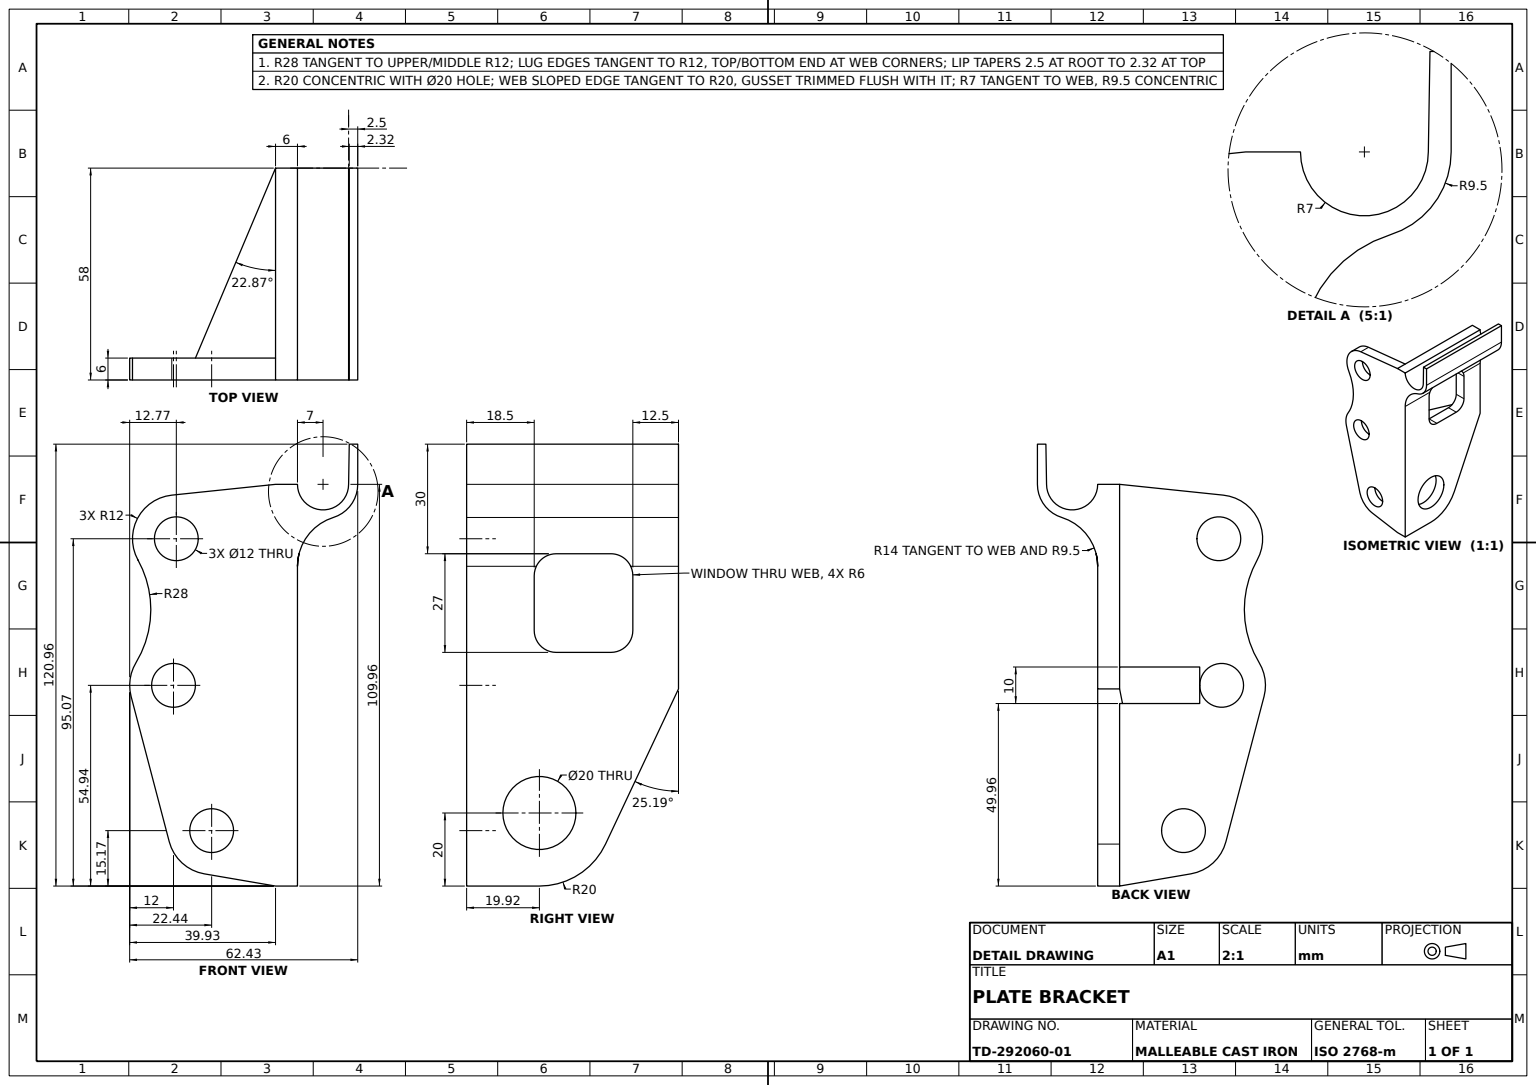
SolidWorks part; units mm, degrees
material "Malleable Cast Iron"
ref_plane "Front Plane" through (0, 0, 0) normal (0, 0, 1) x (1, 0, 0)
ref_plane "Top Plane" through (0, 0, 0) normal (0, 1, 0) x (1, 0, 0)
ref_plane "Right Plane" through (0, 0, 0) normal (1, 0, 0) x (0, 0, -1)
sketch "Base Plate Sketch" plane through (0, 0, 0) normal (0, 0, 1) x (1, 0, 0)
  line L0 (0, 0) -> (58, 0)
  line L1 (58, 0) -> (58, -56)
  line L2 (0, 0) -> (0, -56)
  line L3 (0, -56) -> (58, -56)
  dimension "D1" = 56
  dimension "D2" = 58
extrude "Base Plate" add sketch "Base Plate Sketch" along normal blind 6
sketch "Channel Wall Sketch" plane through (0, 0, 0) normal (-1, 0, 0) x (0, 0, 1)
  line L0 (0, 0) -> (-7, 0)
  line L1 (0, 0) -> (0, -56) construction
  line L2 (-7, 0) -> (-16.5, 0)
  line L3 (0, 0) -> (0, -22.4332)
  arc A1 (-16.5, 0) -> (-9.8298, -9.0688) centre (-7, 0) ccw
  arc A2 (-9.8298, -9.0688) -> (0, -22.4332) centre (-14, -22.4332) cw
  dimension "D2" = 19
  dimension "D3" = 14
  dimension "D4" = 19
  dimension "D7" = 14
  dimension "D6" = 7
extrude "Channel Wall" add sketch "Channel Wall Sketch" against normal blind 58
sketch "Channel Groove Sketch" plane through (0, 0, 0) normal (-1, 0, 0) x (0, 0, 1)
  line L0 (-14, 0) -> (0, 0)
  arc A0 (-14, 0) -> (0, 0) centre (-7, 0) ccw
  dimension "D1" = 14
extrude "Channel Groove Cut" cut sketch "Channel Groove Sketch" against normal blind 58
sketch "Groove Lip Sketch" plane through (0, 0, 0) normal (-1, 0, 0) x (0, 0, 1)
  line L0 (-16.5, 0) -> (-16.5, 11)
  line L1 (-16.5, 11) -> (-14.1792, 11)
  line L2 (-14.1792, 11) -> (-14, 0)
  line L3 (-14, 0) -> (-16.5, 0)
  line L4 (6, 0) -> (0, 0) construction
  dimension "D1" = 4.3495
  dimension "D2" = 11
extrude "Groove Lip" add sketch "Groove Lip Sketch" against normal blind 58
sketch "Side Arm Sketch" plane through (0, 0, 6) normal (0, 0, 1) x (1, 0, 0)
  line L0 (58, 0) -> (58, -109.964)
  line L1 (58, -109.964) -> (38.0764, -109.964)
  line L2 (0, -56) -> (58, -56)
  line L3 (0, -56) -> (19.9783, -98.4763)
  line L4 (0, 0) -> (0, -56) construction
  arc A0 (19.9783, -98.4763) -> (38.0764, -109.964) centre (38.0764, -89.964) ccw
  line M3 (0, -56) -> (58, -56)
  dimension "D1" = 20
  dimension "D2" = 19.9783
  dimension "D3" = 38.0764
extrude "Side Arm" add sketch "Side Arm Sketch" against normal blind 6 contours L3 A0 L1 L0 M3
sketch "Lug Plate Sketch" plane through (58, 0, 0) normal (1, 0, 0) x (0, 0, -1)
  line L1 (-6, -109.964) -> (-25.5178, -106.6187)
  line L2 (-6, 0) -> (-6, -109.964)
  line L5 (-6, 0) -> (-34.4085, -2.9596)
  line L8 (-45.541, -58.0697) -> (-35.097, -97.8392)
  arc A0 (-34.4085, -2.9596) -> (-43.6592, -20.715) centre (-33.165, -14.895) ccw
  arc A1 (-35.097, -97.8392) -> (-25.5178, -106.6187) centre (-23.4905, -94.7912) ccw
  arc A2 (-44.1979, -48.8037) -> (-45.541, -58.0697) centre (-33.9345, -55.0217) ccw
  arc A3 (-43.6592, -20.715) -> (-44.1979, -48.8037) centre (-68.1456, -34.2949) cw
  dimension "D1" = 28
  dimension "D2" = 12
  dimension "D3" = 28
  dimension "D4" = 33.3203
  dimension "D5" = 35.3475
  dimension "D6" = 42.9948
  dimension "D7" = 43.7643
  dimension "D8" = 44.2383
  dimension "D9" = 44.9267
extrude "Lug Plate" add sketch "Lug Plate Sketch" against normal blind 6
sketch "Upper Hole Sketch" plane through (52, 0, 0) normal (-1, 0, 0) x (0, 0, 1)
  circle A0 centre (33.165, -14.895) radius 6
  circle A1 centre (33.9345, -55.0217) radius 6
  circle A2 centre (23.4905, -94.7912) radius 6
  dimension "D1" = 12
  dimension "D2" = 12
  dimension "D3" = 12
  dimension "D4" = 12
  dimension "D5" = 12
  dimension "D6" = 12
extrude "Upper Hole" cut sketch "Upper Hole Sketch" against normal blind 6
sketch "Middle Hole Sketch" plane through (0, 0, 6) normal (0, 0, 1) x (1, 0, 0)
  circle A0 centre (38.0764, -89.964) radius 10
  dimension "D1" = 20
  dimension "D2" = 20
extrude "Middle Hole" cut sketch "Middle Hole Sketch" against normal blind 6
sketch "Gusset Sketch" plane through (0, 0, 0) normal (0, 1, 0) x (1, 0, 0)
  line L0 (52, -6) -> (52, -27.93)
  line L1 (52, -6) -> (52, -34.4085) construction
  line L2 (52, -27.93) -> (0, -6)
  line L3 (0, -6) -> (52, -6)
  line L5 (58, 0) -> (0, 0) construction
  dimension "D1" = 27.93
extrude "Gusset" add sketch "Gusset Sketch" against normal blind 60
sketch "Gusset Trim Sketch A" plane through (0, 0, 0) normal (0, 1, 0) x (1, 0, 0)
  line L0 (0, -6) -> (52, -6)
  line L1 (52, -6) -> (52, -27.93)
  line L2 (52, -27.93) -> (0, -6)
extrude "Gusset Trim Cut A" cut sketch "Gusset Trim Sketch A" against normal blind 50
sketch "Gusset Trim Sketch B" plane through (0, 0, 6) normal (0, 0, -1) x (-1, 0, 0)
  line L0 (-1.8814, -60) -> (0, -56)
  line L1 (0, -56) -> (0, -60)
  line L2 (0, -60) -> (-1.8814, -60)
extrude "Gusset Trim Cut B" cut sketch "Gusset Trim Sketch B" against normal blind 50
sketch "Arm Profile Cut Sketch" plane through (0, 0, 6) normal (0, 0, 1) x (1, 0, 0)
  line L0 (0, 0) -> (0, -50) construction
  line L1 (52, 0) -> (0, 0) construction
  line L3 (18.5, -46) -> (33.5, -46)
  line L4 (12.5, -40) -> (12.5, -25)
  line L5 (18.5, -19) -> (33.5, -19)
  line L6 (39.5, -25) -> (39.5, -40)
  arc A0 (18.5, -46) -> (12.5, -40) centre (18.5, -40) cw
  arc A1 (33.5, -46) -> (39.5, -40) centre (33.5, -40) ccw
  arc A2 (39.5, -25) -> (33.5, -19) centre (33.5, -25) ccw
  arc A3 (12.5, -25) -> (18.5, -19) centre (18.5, -25) cw
  dimension "D1" = 6
  dimension "D4" = 12.5
  dimension "D2" = 15
  dimension "D3" = 27
  dimension "D5" = 19
extrude "Arm Profile Cut" cut sketch "Arm Profile Cut Sketch" against normal blind 6
sketch "Lower Hole Sketch" plane through (0, 0, 0) normal (0, 0, 1) x (1, 0, 0)
  line L0 (13.0767, -22.4332) -> (38.9233, -22.4332)
  line L1 (18.5, -19) -> (33.5, -19)
  arc A0 (18.5, -19) -> (13.0767, -22.4332) centre (18.5, -25) ccw
  arc A1 (38.9233, -22.4332) -> (33.5, -19) centre (33.5, -25) ccw
  dimension "D1" = 12
  dimension "D2" = 12
extrude "Lower Hole" cut sketch "Lower Hole Sketch" against normal blind 6
